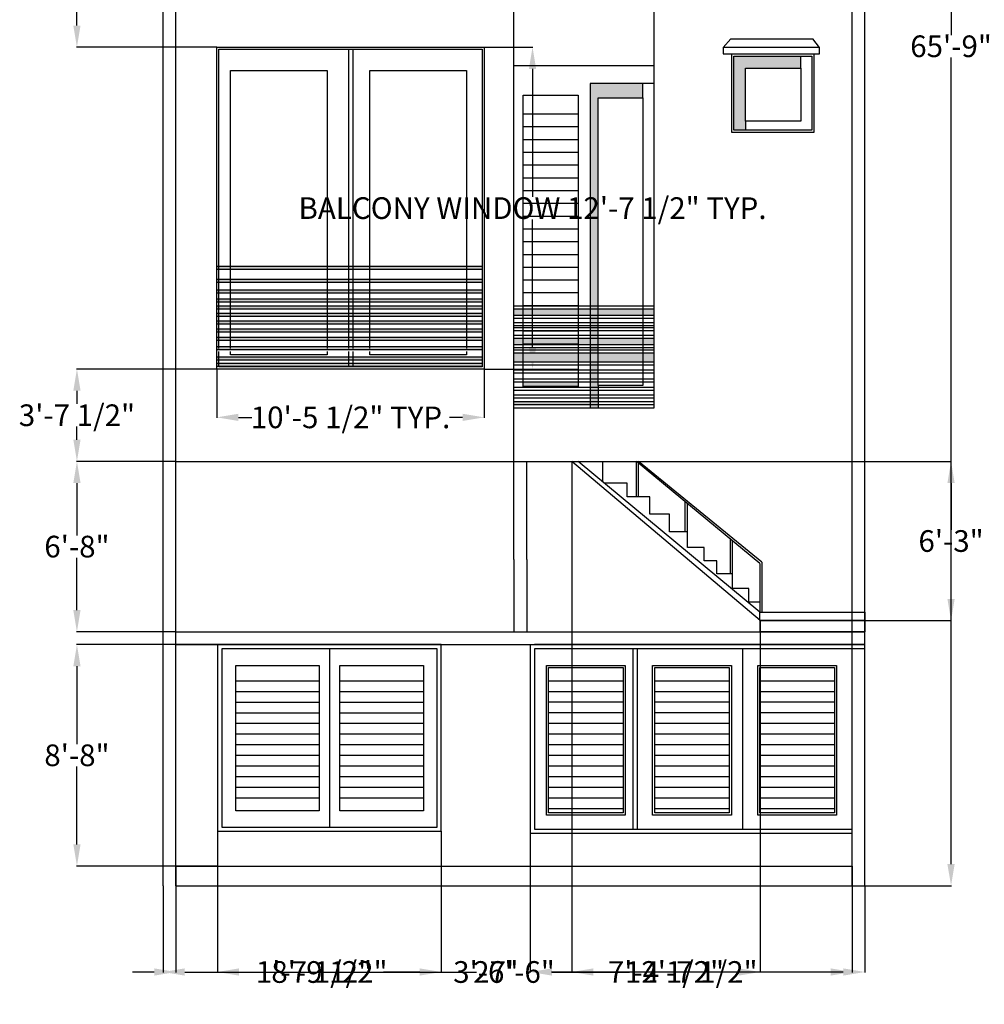
# Model space of a CAD drawing. Units: inches. Extents: x 41 to 5965, y 7 to 3328.
# Tile 4 of 6: x 4990 to 5444, y 2428 to 2890. Entities that reach past the tile are written whole.
import ezdxf

# ---------------------------------------------------------------- set-up
doc = ezdxf.new("R2010")
doc.units = ezdxf.units.IN
doc.header["$MEASUREMENT"] = 0
for name, color, linetype, lineweight in [('A-ANNO-DIMS', 2, 'Continuous', 18), ('A-ELEV', 7, 'Continuous', 25), ('A-ELEV-PATT', 8, 'Continuous', 13)]:
    doc.layers.add(name, color=color, linetype=linetype, lineweight=lineweight)
doc.styles.get("Standard").update_dxf_attribs({"font": 'arial.ttf'})
doc.dimstyles.get("Standard").update_dxf_attribs({"dimtxt": 10.18, "dimasz": 10.18, "dimexe": 0.18, "dimexo": 0.0625, "dimgap": 0.09, "dimtad": 0, "dimtih": 1, "dimtoh": 1, "dimdec": 0, "dimzin": 0, "dimdsep": 46, "dimlunit": 3, "dimtxsty": 'Standard', "dimcen": 0.09, "dimadec": 0, "dimazin": 0, "dimtfac": 1, "dimtdec": 0, "dimtofl": 0, "dimtmove": 0, "dimatfit": 3, "dimfxl": 1, "dimtolj": 1, "dimtzin": 0, "dimarcsym": 0})

# ---------------------------------------------------------------- blocks, each defined once
blk = doc.blocks.new('WIN-ELEV-1')
for p, q in [((0, 0), (0, 151.25)), ((0, 151.25), (125.74, 151.25)), ((1, 150.25), (124.74, 150.25)), ((1, 9.67), (1, 150.25)), ((124.74, 150.25), (124.74, 1)), ((125.74, 151.25), (125.74, 0)), ((1, 1), (1, 8.26)), ((125.74, 0), (0, 0)), ((124.74, 1), (1, 1))]:
    blk.add_line(p, q)
blk = doc.blocks.new('*D32')
at = {"layer": 'A-ANNO-DIMS', "color": 0, "lineweight": -2, "transparency": 16777216}
for p, q in [((5208.81, 2877.58), (5231.61, 2877.58)), ((5231.43, 2867.4), (5231.43, 2807.31)), ((5231.43, 2736.51), (5231.43, 2796.6)), ((5208.81, 2726.33), (5231.61, 2726.33))]:
    blk.add_line(p, q, dxfattribs=at)
at = {"layer": 'A-ANNO-DIMS', "color": 0, "transparency": 16777216}
for points in [[(5229.74, 2867.4), (5233.13, 2867.4), (5231.43, 2877.58)], [(5229.74, 2736.51), (5233.13, 2736.51), (5231.43, 2726.33)]]:
    blk.add_solid(points, dxfattribs=at)
at = {"layer": 'Defpoints', "color": 0, "transparency": 16777216}
for p in [(5208.74, 2877.58), (5231.43, 2877.58), (5208.74, 2726.33)]:
    blk.add_point(p, dxfattribs=at)
at = {"layer": 'A-ANNO-DIMS', "color": 0, "transparency": 16777216, "insert": (5231.43, 2801.96), "char_height": 10.18, "attachment_point": 5}
blk.add_mtext('\\A1;BALCONY WINDOW 12\'-7 1/2" TYP.', dxfattribs=at)
blk = doc.blocks.new('*D33')
at = {"layer": 'A-ANNO-DIMS', "color": 0, "lineweight": -2, "transparency": 16777216}
for p, q in [((5083, 2726.27), (5083, 2703.46)), ((5208.74, 2726.27), (5208.74, 2703.46)), ((5093.18, 2703.64), (5099.42, 2703.64)), ((5198.56, 2703.64), (5192.33, 2703.64))]:
    blk.add_line(p, q, dxfattribs=at)
at = {"layer": 'A-ANNO-DIMS', "color": 0, "transparency": 16777216}
for points in [[(5093.18, 2705.34), (5093.18, 2701.95), (5083, 2703.64)], [(5198.56, 2705.34), (5198.56, 2701.95), (5208.74, 2703.64)]]:
    blk.add_solid(points, dxfattribs=at)
at = {"layer": 'Defpoints', "color": 0, "transparency": 16777216}
for p in [(5083, 2726.33), (5208.74, 2726.33), (5208.74, 2703.64)]:
    blk.add_point(p, dxfattribs=at)
at = {"layer": 'A-ANNO-DIMS', "color": 0, "transparency": 16777216, "insert": (5145.87, 2703.64), "char_height": 10.18, "attachment_point": 5}
blk.add_mtext('\\A1;10\'-5 1/2" TYP.', dxfattribs=at)
blk = doc.blocks.new('*D63')
at = {"layer": 'A-ANNO-DIMS', "color": 0, "lineweight": -2, "transparency": 16777216}
for p, q in [((5057.72, 2483.48), (5057.72, 2442.86)), ((5387.72, 2483.48), (5387.72, 2442.86)), ((5067.9, 2443.04), (5205.06, 2443.04)), ((5377.54, 2443.04), (5240.38, 2443.04))]:
    blk.add_line(p, q, dxfattribs=at)
at = {"layer": 'A-ANNO-DIMS', "color": 0, "transparency": 16777216}
for points in [[(5067.9, 2444.74), (5067.9, 2441.34), (5057.72, 2443.04)], [(5377.54, 2444.74), (5377.54, 2441.34), (5387.72, 2443.04)]]:
    blk.add_solid(points, dxfattribs=at)
at = {"layer": 'Defpoints', "color": 0, "transparency": 16777216}
for p in [(5057.72, 2483.54), (5387.72, 2483.54), (5387.72, 2443.04)]:
    blk.add_point(p, dxfattribs=at)
at = {"layer": 'A-ANNO-DIMS', "color": 0, "transparency": 16777216, "insert": (5222.72, 2443.04), "char_height": 10.18, "attachment_point": 5}
blk.add_mtext('\\A1;27\'-6"', dxfattribs=at)
blk = doc.blocks.new('*D64')
at = {"layer": 'A-ANNO-DIMS', "color": 0, "lineweight": -2, "transparency": 16777216}
for p, q in [((5387.78, 3272.46), (5428.4, 3272.46)), ((5428.22, 3262.28), (5428.22, 2883.29)), ((5428.22, 2493.72), (5428.22, 2872.71)), ((5387.78, 2483.54), (5428.4, 2483.54))]:
    blk.add_line(p, q, dxfattribs=at)
at = {"layer": 'A-ANNO-DIMS', "color": 0, "transparency": 16777216}
for points in [[(5426.52, 3262.28), (5429.92, 3262.28), (5428.22, 3272.46)], [(5426.52, 2493.72), (5429.92, 2493.72), (5428.22, 2483.54)]]:
    blk.add_solid(points, dxfattribs=at)
at = {"layer": 'Defpoints', "color": 0, "transparency": 16777216}
for p in [(5387.72, 3272.46), (5428.22, 3272.46), (5387.72, 2483.54)]:
    blk.add_point(p, dxfattribs=at)
at = {"layer": 'A-ANNO-DIMS', "color": 0, "transparency": 16777216, "insert": (5428.22, 2878), "char_height": 10.18, "attachment_point": 5}
blk.add_mtext('\\A1;65\'-9"', dxfattribs=at)
blk = doc.blocks.new('*D65')
at = {"layer": 'A-ANNO-DIMS', "color": 0, "lineweight": -2, "transparency": 16777216}
for p, q in [((5063.72, 2492.78), (5063.72, 2442.86)), ((5083.3, 2492.78), (5083.3, 2442.86)), ((5053.54, 2443.04), (5043.36, 2443.04)), ((5093.48, 2443.04), (5103.66, 2443.04))]:
    blk.add_line(p, q, dxfattribs=at)
at = {"layer": 'A-ANNO-DIMS', "color": 0, "transparency": 16777216}
for points in [[(5053.54, 2444.74), (5053.54, 2441.34), (5063.72, 2443.04)], [(5093.48, 2444.74), (5093.48, 2441.34), (5083.3, 2443.04)]]:
    blk.add_solid(points, dxfattribs=at)
at = {"layer": 'Defpoints', "color": 0, "transparency": 16777216}
for p in [(5063.72, 2492.84), (5083.3, 2492.84), (5083.3, 2443.04)]:
    blk.add_point(p, dxfattribs=at)
at = {"layer": 'A-ANNO-DIMS', "color": 0, "transparency": 16777216, "insert": (5128.66, 2443.04), "char_height": 10.18, "attachment_point": 5}
blk.add_mtext('\\A1;1\'-7 1/2"', dxfattribs=at)
blk = doc.blocks.new('*D66')
at = {"layer": 'A-ANNO-DIMS', "color": 0, "lineweight": -2, "transparency": 16777216}
for p, q in [((5083.3, 2492.78), (5083.3, 2442.86)), ((5188.55, 2492.78), (5188.55, 2442.86)), ((5093.48, 2443.04), (5110.44, 2443.04)), ((5178.37, 2443.04), (5161.41, 2443.04))]:
    blk.add_line(p, q, dxfattribs=at)
at = {"layer": 'A-ANNO-DIMS', "color": 0, "transparency": 16777216}
for points in [[(5093.48, 2444.74), (5093.48, 2441.34), (5083.3, 2443.04)], [(5178.37, 2444.74), (5178.37, 2441.34), (5188.55, 2443.04)]]:
    blk.add_solid(points, dxfattribs=at)
at = {"layer": 'Defpoints', "color": 0, "transparency": 16777216}
for p in [(5083.3, 2492.84), (5188.55, 2492.84), (5188.55, 2443.04)]:
    blk.add_point(p, dxfattribs=at)
at = {"layer": 'A-ANNO-DIMS', "color": 0, "transparency": 16777216, "insert": (5135.93, 2443.04), "char_height": 10.18, "attachment_point": 5}
blk.add_mtext('\\A1;8\'-9 1/2"', dxfattribs=at)
blk = doc.blocks.new('*D67')
at = {"layer": 'A-ANNO-DIMS', "color": 0, "lineweight": -2, "transparency": 16777216}
for p, q in [((5188.55, 2492.78), (5188.55, 2442.86)), ((5230.39, 2492.78), (5230.39, 2442.86)), ((5178.37, 2443.04), (5168.19, 2443.04)), ((5240.57, 2443.04), (5250.75, 2443.04))]:
    blk.add_line(p, q, dxfattribs=at)
at = {"layer": 'A-ANNO-DIMS', "color": 0, "transparency": 16777216}
for points in [[(5178.37, 2444.74), (5178.37, 2441.34), (5188.55, 2443.04)], [(5240.57, 2444.74), (5240.57, 2441.34), (5230.39, 2443.04)]]:
    blk.add_solid(points, dxfattribs=at)
at = {"layer": 'Defpoints', "color": 0, "transparency": 16777216}
for p in [(5188.55, 2492.84), (5230.39, 2492.84), (5230.39, 2443.04)]:
    blk.add_point(p, dxfattribs=at)
at = {"layer": 'A-ANNO-DIMS', "color": 0, "transparency": 16777216, "insert": (5209.47, 2443.04), "char_height": 10.18, "attachment_point": 5}
blk.add_mtext('\\A1;3\'-6"', dxfattribs=at)
blk = doc.blocks.new('*D68')
at = {"layer": 'A-ANNO-DIMS', "color": 0, "lineweight": -2, "transparency": 16777216}
for p, q in [((5230.39, 2492.78), (5230.39, 2442.86)), ((5381.72, 2492.78), (5381.72, 2442.86)), ((5240.57, 2443.04), (5277.1, 2443.04)), ((5371.54, 2443.04), (5335.01, 2443.04))]:
    blk.add_line(p, q, dxfattribs=at)
at = {"layer": 'A-ANNO-DIMS', "color": 0, "transparency": 16777216}
for points in [[(5240.57, 2444.74), (5240.57, 2441.34), (5230.39, 2443.04)], [(5371.54, 2444.74), (5371.54, 2441.34), (5381.72, 2443.04)]]:
    blk.add_solid(points, dxfattribs=at)
at = {"layer": 'Defpoints', "color": 0, "transparency": 16777216}
for p in [(5230.39, 2492.84), (5381.72, 2492.84), (5381.72, 2443.04)]:
    blk.add_point(p, dxfattribs=at)
at = {"layer": 'A-ANNO-DIMS', "color": 0, "transparency": 16777216, "insert": (5306.06, 2443.04), "char_height": 10.18, "attachment_point": 5}
blk.add_mtext('\\A1;12\'-7 1/2"', dxfattribs=at)
blk = doc.blocks.new('*D69')
at = {"layer": 'A-ANNO-DIMS', "color": 0, "lineweight": -2, "transparency": 16777216}
for p, q in [((5083.23, 2596.88), (5017.04, 2596.88)), ((5017.22, 2586.7), (5017.22, 2550.15)), ((5017.22, 2503.02), (5017.22, 2539.57)), ((5083.23, 2492.84), (5017.04, 2492.84))]:
    blk.add_line(p, q, dxfattribs=at)
at = {"layer": 'A-ANNO-DIMS', "color": 0, "transparency": 16777216}
for points in [[(5015.52, 2586.7), (5018.92, 2586.7), (5017.22, 2596.88)], [(5015.52, 2503.02), (5018.92, 2503.02), (5017.22, 2492.84)]]:
    blk.add_solid(points, dxfattribs=at)
at = {"layer": 'Defpoints', "color": 0, "transparency": 16777216}
for p in [(5017.22, 2596.88), (5083.3, 2596.88), (5083.3, 2492.84)]:
    blk.add_point(p, dxfattribs=at)
at = {"layer": 'A-ANNO-DIMS', "color": 0, "transparency": 16777216, "insert": (5017.22, 2544.86), "char_height": 10.18, "attachment_point": 5}
blk.add_mtext('\\A1;8\'-8"', dxfattribs=at)
blk = doc.blocks.new('*D70')
at = {"layer": 'A-ANNO-DIMS', "color": 0, "lineweight": -2, "transparency": 16777216}
for p, q in [((5063.66, 2682.95), (5017.04, 2682.95)), ((5017.22, 2672.77), (5017.22, 2648.2)), ((5017.22, 2613.06), (5017.22, 2637.63)), ((5063.66, 2602.88), (5017.04, 2602.88))]:
    blk.add_line(p, q, dxfattribs=at)
at = {"layer": 'A-ANNO-DIMS', "color": 0, "transparency": 16777216}
for points in [[(5015.52, 2672.77), (5018.92, 2672.77), (5017.22, 2682.95)], [(5015.52, 2613.06), (5018.92, 2613.06), (5017.22, 2602.88)]]:
    blk.add_solid(points, dxfattribs=at)
at = {"layer": 'Defpoints', "color": 0, "transparency": 16777216}
for p in [(5017.22, 2682.95), (5063.72, 2682.95), (5063.72, 2602.88)]:
    blk.add_point(p, dxfattribs=at)
at = {"layer": 'A-ANNO-DIMS', "color": 0, "transparency": 16777216, "insert": (5017.22, 2642.92), "char_height": 10.18, "attachment_point": 5}
blk.add_mtext('\\A1;6\'-8"', dxfattribs=at)
blk = doc.blocks.new('*D71')
at = {"layer": 'A-ANNO-DIMS', "color": 0, "lineweight": -2, "transparency": 16777216}
for p, q in [((5082.94, 2726.33), (5017.04, 2726.33)), ((5017.22, 2716.15), (5017.22, 2710)), ((5017.22, 2693.13), (5017.22, 2699.28)), ((5063.66, 2682.95), (5017.04, 2682.95))]:
    blk.add_line(p, q, dxfattribs=at)
at = {"layer": 'A-ANNO-DIMS', "color": 0, "transparency": 16777216}
for points in [[(5015.52, 2716.15), (5018.92, 2716.15), (5017.22, 2726.33)], [(5015.52, 2693.13), (5018.92, 2693.13), (5017.22, 2682.95)]]:
    blk.add_solid(points, dxfattribs=at)
at = {"layer": 'Defpoints', "color": 0, "transparency": 16777216}
for p in [(5017.22, 2726.33), (5083, 2726.33), (5063.72, 2682.95)]:
    blk.add_point(p, dxfattribs=at)
at = {"layer": 'A-ANNO-DIMS', "color": 0, "transparency": 16777216, "insert": (5017.22, 2704.64), "char_height": 10.18, "attachment_point": 5}
blk.add_mtext('\\A1;3\'-7 1/2"', dxfattribs=at)
blk = doc.blocks.new('*D72')
at = {"layer": 'A-ANNO-DIMS', "color": 0, "lineweight": -2, "transparency": 16777216}
for p, q in [((5079.42, 2985.67), (5017.04, 2985.67)), ((5017.22, 2975.49), (5017.22, 2936.92)), ((5017.22, 2887.76), (5017.22, 2926.34)), ((5082.94, 2877.58), (5017.04, 2877.58))]:
    blk.add_line(p, q, dxfattribs=at)
at = {"layer": 'A-ANNO-DIMS', "color": 0, "transparency": 16777216}
for points in [[(5015.52, 2975.49), (5018.92, 2975.49), (5017.22, 2985.67)], [(5015.52, 2887.76), (5018.92, 2887.76), (5017.22, 2877.58)]]:
    blk.add_solid(points, dxfattribs=at)
at = {"layer": 'Defpoints', "color": 0, "transparency": 16777216}
for p in [(5017.22, 2985.67), (5079.49, 2985.67), (5083, 2877.58)]:
    blk.add_point(p, dxfattribs=at)
at = {"layer": 'A-ANNO-DIMS', "color": 0, "transparency": 16777216, "insert": (5017.22, 2931.63), "char_height": 10.18, "attachment_point": 5}
blk.add_mtext('\\A1;9\'-0"', dxfattribs=at)
blk = doc.blocks.new('*D77')
at = {"layer": 'A-ANNO-DIMS', "color": 0, "lineweight": -2, "transparency": 16777216}
for p, q in [((5249.9, 2682.89), (5249.9, 2442.86)), ((5338.47, 2608.06), (5338.47, 2442.86)), ((5260.08, 2443.04), (5268.75, 2443.04)), ((5328.29, 2443.04), (5319.63, 2443.04))]:
    blk.add_line(p, q, dxfattribs=at)
at = {"layer": 'A-ANNO-DIMS', "color": 0, "transparency": 16777216}
for points in [[(5260.08, 2444.74), (5260.08, 2441.34), (5249.9, 2443.04)], [(5328.29, 2444.74), (5328.29, 2441.34), (5338.47, 2443.04)]]:
    blk.add_solid(points, dxfattribs=at)
at = {"layer": 'Defpoints', "color": 0, "transparency": 16777216}
for p in [(5249.9, 2682.95), (5338.47, 2608.13), (5338.47, 2443.04)]:
    blk.add_point(p, dxfattribs=at)
at = {"layer": 'A-ANNO-DIMS', "color": 0, "transparency": 16777216, "insert": (5294.19, 2443.04), "char_height": 10.18, "attachment_point": 5}
blk.add_mtext('\\A1;7\'-4 1/2"', dxfattribs=at)
blk = doc.blocks.new('*D78')
at = {"layer": 'A-ANNO-DIMS', "color": 0, "lineweight": -2, "transparency": 16777216}
for p, q in [((5249.96, 2682.95), (5428.4, 2682.95)), ((5428.22, 2672.77), (5428.22, 2650.83)), ((5428.22, 2618.31), (5428.22, 2640.25)), ((5338.54, 2608.13), (5428.4, 2608.13))]:
    blk.add_line(p, q, dxfattribs=at)
at = {"layer": 'A-ANNO-DIMS', "color": 0, "transparency": 16777216}
for points in [[(5426.52, 2672.77), (5429.92, 2672.77), (5428.22, 2682.95)], [(5426.52, 2618.31), (5429.92, 2618.31), (5428.22, 2608.13)]]:
    blk.add_solid(points, dxfattribs=at)
at = {"layer": 'Defpoints', "color": 0, "transparency": 16777216}
for p in [(5249.9, 2682.95), (5338.47, 2608.13), (5428.22, 2608.13)]:
    blk.add_point(p, dxfattribs=at)
at = {"layer": 'A-ANNO-DIMS', "color": 0, "transparency": 16777216, "insert": (5428.22, 2645.54), "char_height": 10.18, "attachment_point": 5}
blk.add_mtext('\\A1;6\'-3"', dxfattribs=at)

msp = doc.modelspace()

# ---------------------------------------------------------------- hatches: boundary and pattern name
at = {"layer": 'A-ELEV-PATT'}
h = msp.add_hatch(color=256, dxfattribs=at)
h.dxf.hatch_style = 1
h.paths.add_polyline_path([(5326.1, 2838.56), (5331.59, 2838.56), (5331.59, 2842.77), (5331.59, 2867.75), (5357.62, 2867.75), (5357.62, 2873.38), (5326.1, 2873.38)])
h = msp.add_hatch(color=256, dxfattribs=at)
h.dxf.hatch_style = 1
h.paths.add_polyline_path([(5283.31, 2860.46), (5258.54, 2860.46), (5258.54, 2708.16), (5262.29, 2708.16), (5262.29, 2718.67), (5262.29, 2853.73), (5283.31, 2853.73)])
h = msp.add_hatch(color=256, dxfattribs=at)
h.dxf.hatch_style = 1
h.paths.add_polyline_path([(5207.74, 2774.65), (5083, 2774.65), (5083, 2773.25), (5207.74, 2773.25)])
h = msp.add_hatch(color=256, dxfattribs=at)
h.dxf.hatch_style = 1
h.paths.add_polyline_path([(5207.74, 2768.59), (5083, 2768.59), (5083, 2767.18), (5207.74, 2767.18)])
h = msp.add_hatch(color=256, dxfattribs=at)
h.dxf.hatch_style = 1
h.paths.add_polyline_path([(5207.74, 2763.59), (5083, 2763.59), (5083, 2762.18), (5207.74, 2762.18)])
h = msp.add_hatch(color=256, dxfattribs=at)
h.dxf.hatch_style = 1
h.paths.add_polyline_path([(5207.74, 2759.3), (5083, 2759.3), (5083, 2757.89), (5207.74, 2757.89)])
h = msp.add_hatch(color=256, dxfattribs=at)
h.dxf.hatch_style = 1
h.paths.add_polyline_path([(5207.74, 2756.07), (5083, 2756.07), (5083, 2754.67), (5207.74, 2754.67)])
h = msp.add_hatch(color=256, dxfattribs=at)
h.dxf.hatch_style = 1
h.paths.add_polyline_path([(5252.94, 2740.84), (5227.05, 2740.84), (5227.05, 2738.24), (5252.94, 2738.24)])
h.paths.add_polyline_path([(5227.05, 2740.84), (5222.72, 2740.84), (5222.72, 2737.95), (5227.05, 2737.95)])
h.paths.add_polyline_path([(5283.31, 2740.84), (5262.29, 2740.84), (5262.29, 2737.95), (5283.31, 2737.95)])
h.paths.add_polyline_path([(5258.54, 2740.84), (5252.94, 2740.84), (5252.94, 2737.95), (5258.54, 2737.95)])
h.paths.add_polyline_path([(5288.65, 2740.84), (5283.31, 2740.84), (5283.31, 2737.95), (5288.65, 2737.95)])
h.paths.add_polyline_path([(5283.31, 2754.66), (5262.29, 2754.66), (5262.29, 2751.62), (5283.31, 2751.62)])
h.paths.add_polyline_path([(5252.94, 2754.66), (5227.05, 2754.66), (5227.05, 2751.62), (5252.94, 2751.62)])
h.paths.add_polyline_path([(5258.54, 2754.66), (5252.94, 2754.66), (5252.94, 2751.62), (5258.54, 2751.62)])
h.paths.add_polyline_path([(5288.65, 2754.66), (5283.31, 2754.66), (5283.31, 2751.62), (5288.65, 2751.62)])
h.paths.add_polyline_path([(5227.05, 2754.66), (5222.72, 2754.66), (5222.72, 2751.62), (5227.05, 2751.62)])
h.paths.add_polyline_path([(5283.31, 2733.93), (5262.29, 2733.93), (5262.29, 2729.81), (5283.31, 2729.81)])
h = msp.add_hatch(color=256, dxfattribs=at)
h.dxf.hatch_style = 1
h.paths.add_polyline_path([(5207.74, 2752.65), (5083, 2752.65), (5083, 2751.24), (5207.74, 2751.24)])
h = msp.add_hatch(color=256, dxfattribs=at)
h.dxf.hatch_style = 1
h.paths.add_polyline_path([(5207.74, 2748.99), (5083, 2748.99), (5083, 2747.59), (5207.74, 2747.59)])
h = msp.add_hatch(color=256, dxfattribs=at)
h.dxf.hatch_style = 1
h.paths.add_polyline_path([(5207.74, 2745.19), (5083, 2745.19), (5083, 2743.79), (5207.74, 2743.79)])
h = msp.add_hatch(color=256, dxfattribs=at)
h.dxf.hatch_style = 1
h.paths.add_polyline_path([(5207.74, 2741.28), (5083, 2741.28), (5083, 2739.87), (5207.74, 2739.87)])
h = msp.add_hatch(color=256, dxfattribs=at)
h.dxf.hatch_style = 1
h.paths.add_polyline_path([(5207.74, 2737), (5083, 2737), (5083, 2735.59), (5207.74, 2735.59)])
h = msp.add_hatch(color=256, dxfattribs=at)
h.dxf.hatch_style = 1
h.paths.add_polyline_path([(5207.74, 2732.1), (5083, 2732.1), (5083, 2730.69), (5207.74, 2730.69)])
h = msp.add_hatch(color=256, dxfattribs=at)
h.dxf.hatch_style = 1
h.paths.add_polyline_path([(5252.94, 2733.93), (5227.05, 2733.93), (5227.05, 2729.81), (5252.94, 2729.81)])
h.paths.add_polyline_path([(5227.05, 2733.93), (5222.72, 2733.93), (5222.72, 2729.81), (5227.05, 2729.81)])
h.paths.add_polyline_path([(5258.54, 2733.93), (5252.94, 2733.93), (5252.94, 2729.81), (5258.54, 2729.81)])
h.paths.add_polyline_path([(5288.65, 2733.93), (5283.31, 2733.93), (5283.31, 2729.81), (5288.65, 2729.81)])
h.paths.add_polyline_path([(5252.94, 2720.41), (5227.05, 2720.41), (5227.05, 2718.13), (5252.94, 2718.13)])
h.paths.add_polyline_path([(5258.54, 2711.07), (5222.72, 2711.07), (5222.72, 2709.66), (5258.54, 2709.66)])
h = msp.add_hatch(color=256, dxfattribs=at)
h.dxf.hatch_style = 1
h.paths.add_polyline_path([(5207.74, 2729.18), (5083, 2729.18), (5083, 2727.77), (5207.74, 2727.77)])

# ---------------------------------------------------------------- linework, layer by layer
at = {"layer": 'A-ELEV'}
for p, q in [((5057.72, 2483.54), (5057.72, 3272.46)), ((5222.72, 2682.95), (5222.72, 3272.46)), ((5288.65, 2708.16), (5288.65, 3272.46)), ((5381.72, 2483.54), (5381.72, 3272.46)), ((5387.72, 2483.54), (5387.72, 3272.46)), ((5063.72, 2483.54), (5063.72, 3263.67)), ((5321.09, 2877.43), (5324.61, 2881.49)), ((5324.61, 2881.49), (5363.21, 2881.49)), ((5366.37, 2877.43), (5363.21, 2881.49)), ((5144.87, 2876.58), (5144.87, 2736)), ((5146.87, 2876.58), (5146.87, 2736)), ((5357.62, 2867.75), (5357.62, 2873.38)), ((5222.72, 2868.96), (5288.65, 2868.96)), ((5288.65, 2860.46), (5258.54, 2860.46)), ((5258.54, 2860.46), (5258.54, 2708.16)), ((5283.31, 2853.73), (5283.31, 2860.46)), ((5227.05, 2846.24), (5252.94, 2846.24)), ((5331.59, 2842.77), (5331.59, 2838.56)), ((5227.05, 2840.24), (5252.94, 2840.24)), ((5227.05, 2834.24), (5252.94, 2834.24)), ((5227.05, 2828.24), (5252.94, 2828.24)), ((5227.05, 2822.24), (5252.94, 2822.24)), ((5227.05, 2816.24), (5252.94, 2816.24)), ((5227.05, 2810.24), (5252.94, 2810.24)), ((5227.05, 2804.24), (5252.94, 2804.24)), ((5227.05, 2798.24), (5252.94, 2798.24)), ((5227.05, 2792.24), (5252.94, 2792.24)), ((5227.05, 2786.24), (5252.94, 2786.24)), ((5227.05, 2780.24), (5252.94, 2780.24)), ((5083, 2774.65), (5207.74, 2774.65)), ((5083, 2773.25), (5207.74, 2773.25)), ((5227.05, 2774.24), (5252.94, 2774.24)), ((5083, 2768.59), (5207.74, 2768.59)), ((5083, 2767.18), (5207.74, 2767.18)), ((5227.05, 2768.24), (5252.94, 2768.24)), ((5083, 2763.59), (5207.74, 2763.59)), ((5083, 2762.18), (5207.74, 2762.18)), ((5227.05, 2762.24), (5252.94, 2762.24)), ((5083, 2759.3), (5207.74, 2759.3)), ((5083, 2757.89), (5207.74, 2757.89)), ((5083, 2756.07), (5207.74, 2756.07)), ((5083, 2754.67), (5207.74, 2754.67)), ((5222.72, 2756.07), (5288.65, 2756.07)), ((5222.72, 2754.66), (5288.65, 2754.66)), ((5227.05, 2756.24), (5252.94, 2756.24)), ((5083, 2752.65), (5207.74, 2752.65)), ((5083, 2751.24), (5207.74, 2751.24)), ((5083, 2748.99), (5207.74, 2748.99)), ((5222.72, 2751.62), (5288.65, 2751.62)), ((5222.72, 2750.21), (5288.65, 2750.21)), ((5222.72, 2748.24), (5288.65, 2748.24)), ((5227.05, 2750.24), (5252.94, 2750.24)), ((5083, 2747.59), (5207.74, 2747.59)), ((5083, 2745.19), (5207.74, 2745.19)), ((5083, 2743.79), (5207.74, 2743.79)), ((5222.72, 2746.83), (5288.65, 2746.83)), ((5222.72, 2745.94), (5288.65, 2745.94)), ((5222.72, 2744.53), (5288.65, 2744.53)), ((5227.05, 2744.24), (5252.94, 2744.24)), ((5083, 2741.28), (5207.74, 2741.28)), ((5083, 2739.87), (5207.74, 2739.87)), ((5222.72, 2742.25), (5288.65, 2742.25)), ((5222.72, 2740.84), (5288.65, 2740.84)), ((5083, 2737), (5207.74, 2737)), ((5083, 2735.59), (5207.74, 2735.59)), ((5144.87, 2734.59), (5144.87, 2727.33)), ((5146.87, 2734.59), (5146.87, 2727.33)), ((5222.72, 2737.95), (5288.65, 2737.95)), ((5222.72, 2736.54), (5288.65, 2736.54)), ((5222.72, 2735.34), (5288.65, 2735.34)), ((5227.05, 2738.24), (5252.94, 2738.24)), ((5083, 2732.1), (5207.74, 2732.1)), ((5083, 2730.69), (5207.74, 2730.69)), ((5222.72, 2733.93), (5288.65, 2733.93)), ((5222.72, 2729.81), (5288.65, 2729.81)), ((5083, 2729.18), (5207.74, 2729.18)), ((5083, 2727.77), (5207.74, 2727.77)), ((5222.72, 2728.4), (5288.65, 2728.4)), ((5222.72, 2725.97), (5288.65, 2725.97)), ((5227.05, 2726.24), (5252.94, 2726.24)), ((5222.72, 2724.56), (5288.65, 2724.56)), ((5222.72, 2721.82), (5288.65, 2721.82)), ((5222.72, 2720.41), (5288.65, 2720.41)), ((5222.72, 2717.83), (5288.65, 2717.83)), ((5222.72, 2716.42), (5288.65, 2716.42)), ((5262.29, 2718.67), (5262.29, 2708.16)), ((5222.72, 2714.3), (5288.65, 2714.3)), ((5222.72, 2712.89), (5288.65, 2712.89)), ((5222.72, 2711.07), (5288.65, 2711.07)), ((5222.72, 2709.66), (5288.65, 2709.66)), ((5222.72, 2708.16), (5288.65, 2708.16)), ((5063.72, 2682.95), (5387.72, 2682.95)), ((5222.72, 2636.84), (5222.72, 2682.95)), ((5228.72, 2636.84), (5228.72, 2682.95)), ((5338.47, 2608.13), (5249.9, 2682.95)), ((5338.25, 2612.15), (5252.82, 2682.95)), ((5264.53, 2673.25), (5264.53, 2682.95)), ((5280.26, 2666.28), (5280.26, 2682.95)), ((5338.25, 2635.02), (5280.26, 2682.95)), ((5281.26, 2666.28), (5281.26, 2682.95)), ((5339.32, 2635.64), (5281.26, 2682.95)), ((5303.25, 2682.95), (5303.25, 2683.13)), ((5304.25, 2682.95), (5304.25, 2683.13)), ((5275.92, 2672.69), (5265.2, 2672.69)), ((5275.92, 2666.28), (5275.92, 2672.69)), ((5286.61, 2666.28), (5275.92, 2666.28)), ((5286.61, 2658.22), (5286.61, 2666.28)), ((5303.25, 2649.82), (5303.25, 2663.95)), ((5304.25, 2649.82), (5304.25, 2663.13)), ((5295.88, 2658.22), (5286.61, 2658.22)), ((5295.88, 2649.82), (5295.88, 2658.22)), ((5304.25, 2649.82), (5295.88, 2649.82)), ((5304.25, 2642.56), (5304.25, 2649.82)), ((5324.51, 2630.09), (5324.51, 2646.38)), ((5312.16, 2642.56), (5304.25, 2642.56)), ((5312.16, 2636.25), (5312.16, 2642.56)), ((5325.51, 2630.09), (5325.51, 2645.55)), ((5222.72, 2636.84), (5222.72, 2602.88)), ((5228.72, 2636.84), (5228.72, 2602.88)), ((5318.05, 2636.25), (5312.16, 2636.25)), ((5318.05, 2630.09), (5318.05, 2636.25)), ((5338.25, 2635.02), (5338.25, 2612.15)), ((5339.32, 2635.64), (5339.32, 2612.15)), ((5325.51, 2630.09), (5318.05, 2630.09)), ((5325.51, 2623.21), (5325.51, 2630.09)), ((5333.11, 2623.21), (5325.51, 2623.21)), ((5333.11, 2616.77), (5333.11, 2623.21)), ((5338.25, 2616.77), (5333.11, 2616.77)), ((5063.72, 2602.88), (5387.72, 2602.88)), ((5063.72, 2596.88), (5387.72, 2596.88)), ((5083.3, 2596.88), (5083.3, 2509.14)), ((5188.55, 2596.88), (5083.3, 2596.88)), ((5188.55, 2509.14), (5188.55, 2596.88)), ((5230.39, 2596.88), (5230.39, 2492.84)), ((5387.72, 2596.88), (5232.39, 2596.88)), ((5085.3, 2594.88), (5085.3, 2511.14)), ((5186.55, 2594.88), (5085.3, 2594.88)), ((5135.93, 2594.88), (5135.93, 2511.14)), ((5186.55, 2511.14), (5186.55, 2594.88)), ((5232.39, 2594.88), (5232.39, 2510.22)), ((5387.72, 2594.88), (5232.39, 2594.88)), ((5278.76, 2510.22), (5278.76, 2594.88)), ((5280.76, 2510.22), (5280.76, 2594.88)), ((5330.17, 2594.88), (5330.17, 2510.22)), ((5381.72, 2483.54), (5381.72, 2594.88)), ((5381.72, 2508.22), (5381.72, 2594.88)), ((5381.72, 2492.84), (5381.72, 2594.88)), ((5091.87, 2579.88), (5131.15, 2579.88)), ((5140.86, 2579.88), (5180.14, 2579.88)), ((5238.99, 2579.91), (5274.06, 2579.91)), ((5288.88, 2579.91), (5323.94, 2579.91)), ((5338.3, 2579.91), (5373.36, 2579.91)), ((5091.87, 2574.88), (5131.15, 2574.88)), ((5140.86, 2574.88), (5180.14, 2574.88)), ((5238.99, 2574.91), (5274.06, 2574.91)), ((5288.88, 2574.91), (5323.94, 2574.91)), ((5338.3, 2574.91), (5373.36, 2574.91)), ((5091.87, 2569.88), (5131.15, 2569.88)), ((5140.86, 2569.88), (5180.14, 2569.88)), ((5238.99, 2569.91), (5274.06, 2569.91)), ((5288.88, 2569.91), (5323.94, 2569.91)), ((5338.3, 2569.91), (5373.36, 2569.91)), ((5091.87, 2564.88), (5131.15, 2564.88)), ((5140.86, 2564.88), (5180.14, 2564.88)), ((5238.99, 2564.91), (5274.06, 2564.91)), ((5288.88, 2564.91), (5323.94, 2564.91)), ((5338.3, 2564.91), (5373.36, 2564.91)), ((5091.87, 2559.88), (5131.15, 2559.88)), ((5140.86, 2559.88), (5180.14, 2559.88)), ((5238.99, 2559.91), (5274.06, 2559.91)), ((5288.88, 2559.91), (5323.94, 2559.91)), ((5338.3, 2559.91), (5373.36, 2559.91)), ((5091.87, 2554.88), (5131.15, 2554.88)), ((5140.86, 2554.88), (5180.14, 2554.88)), ((5238.99, 2554.91), (5274.06, 2554.91)), ((5288.88, 2554.91), (5323.94, 2554.91)), ((5338.3, 2554.91), (5373.36, 2554.91)), ((5091.87, 2549.88), (5131.15, 2549.88)), ((5140.86, 2549.88), (5180.14, 2549.88)), ((5238.99, 2549.91), (5274.06, 2549.91)), ((5288.88, 2549.91), (5323.94, 2549.91)), ((5338.3, 2549.91), (5373.36, 2549.91)), ((5091.87, 2544.88), (5131.15, 2544.88)), ((5140.86, 2544.88), (5180.14, 2544.88)), ((5238.99, 2544.91), (5274.06, 2544.91)), ((5288.88, 2544.91), (5323.94, 2544.91)), ((5338.3, 2544.91), (5373.36, 2544.91)), ((5091.87, 2539.88), (5131.15, 2539.88)), ((5140.86, 2539.88), (5180.14, 2539.88)), ((5238.99, 2539.91), (5274.06, 2539.91)), ((5288.88, 2539.91), (5323.94, 2539.91)), ((5338.3, 2539.91), (5373.36, 2539.91)), ((5091.87, 2534.88), (5131.15, 2534.88)), ((5140.86, 2534.88), (5180.14, 2534.88)), ((5238.99, 2534.91), (5274.06, 2534.91)), ((5288.88, 2534.91), (5323.94, 2534.91)), ((5338.3, 2534.91), (5373.36, 2534.91)), ((5091.87, 2529.88), (5131.15, 2529.88)), ((5140.86, 2529.88), (5180.14, 2529.88)), ((5238.99, 2529.91), (5274.06, 2529.91)), ((5288.88, 2529.91), (5323.94, 2529.91)), ((5338.3, 2529.91), (5373.36, 2529.91)), ((5091.87, 2524.88), (5131.15, 2524.88)), ((5140.86, 2524.88), (5180.14, 2524.88)), ((5238.99, 2524.91), (5274.06, 2524.91)), ((5288.88, 2524.91), (5323.94, 2524.91)), ((5338.3, 2524.91), (5373.36, 2524.91)), ((5063.72, 2483.54), (5063.72, 2519.54)), ((5238.99, 2519.91), (5274.06, 2519.91)), ((5288.88, 2519.91), (5323.94, 2519.91)), ((5338.3, 2519.91), (5373.36, 2519.91)), ((5083.3, 2509.14), (5188.55, 2509.14)), ((5083.3, 2509.14), (5083.3, 2492.84)), ((5085.3, 2511.14), (5186.55, 2511.14)), ((5188.55, 2509.14), (5188.55, 2492.84)), ((5230.39, 2508.22), (5381.72, 2508.22)), ((5232.39, 2510.22), (5381.72, 2510.22)), ((5063.72, 2492.84), (5381.72, 2492.84)), ((5063.72, 2483.54), (5387.72, 2483.54))]:
    msp.add_line(p, q, dxfattribs=at)
for points in [[(5321.09, 2874.38), (5321.09, 2874.38), (5366.37, 2874.38), (5366.37, 2874.38), (5366.37, 2877.43), (5366.37, 2877.43), (5321.09, 2877.43), (5321.09, 2877.43)], [(5325.1, 2874.38), (5325.1, 2874.38), (5363.69, 2874.38), (5363.69, 2874.38), (5363.69, 2837.56), (5363.69, 2837.56), (5325.1, 2837.56), (5325.1, 2837.56)], [(5326.1, 2873.38), (5362.69, 2873.38), (5362.69, 2838.56), (5326.1, 2838.56)], [(5331.59, 2867.75), (5331.59, 2867.75), (5357.62, 2867.75), (5357.62, 2867.75), (5357.62, 2842.77), (5357.62, 2842.77), (5331.59, 2842.77), (5331.59, 2842.77)], [(5227.05, 2855), (5227.05, 2855), (5252.94, 2855), (5252.94, 2855), (5252.94, 2718.13), (5252.94, 2718.13), (5227.05, 2718.13), (5227.05, 2718.13)], [(5262.29, 2853.73), (5262.29, 2853.73), (5283.31, 2853.73), (5283.31, 2853.73), (5283.31, 2718.67), (5283.31, 2718.67), (5262.29, 2718.67), (5262.29, 2718.67)], [(5387.72, 2608.13), (5387.72, 2608.13), (5338.25, 2608.13), (5338.25, 2608.13), (5338.25, 2612.15), (5338.25, 2612.15), (5387.72, 2612.15), (5387.72, 2612.15)], [(5387.72, 2602.88), (5387.72, 2602.88), (5338.47, 2602.88), (5338.47, 2602.88), (5338.47, 2608.13), (5338.47, 2608.13), (5387.72, 2608.13), (5387.72, 2608.13)], [(5091.87, 2587.07), (5091.87, 2587.07), (5131.15, 2587.07), (5131.15, 2587.07), (5131.15, 2518.75), (5131.15, 2518.75), (5091.87, 2518.75), (5091.87, 2518.75)], [(5140.86, 2587.07), (5140.86, 2587.07), (5180.14, 2587.07), (5180.14, 2587.07), (5180.14, 2518.75), (5180.14, 2518.75), (5140.86, 2518.75), (5140.86, 2518.75)], [(5237.99, 2587.07), (5237.99, 2587.07), (5275.06, 2587.07), (5275.06, 2587.07), (5275.06, 2516.76), (5275.06, 2516.76), (5237.99, 2516.76), (5237.99, 2516.76)], [(5287.88, 2587.07), (5287.88, 2587.07), (5324.94, 2587.07), (5324.94, 2587.07), (5324.94, 2516.76), (5324.94, 2516.76), (5287.88, 2516.76), (5287.88, 2516.76)], [(5337.3, 2587.07), (5337.3, 2587.07), (5374.36, 2587.07), (5374.36, 2587.07), (5374.36, 2516.76), (5374.36, 2516.76), (5337.3, 2516.76), (5337.3, 2516.76)], [(5238.99, 2586.07), (5274.06, 2586.07), (5274.06, 2517.76), (5238.99, 2517.76)], [(5288.88, 2586.07), (5323.94, 2586.07), (5323.94, 2517.76), (5288.88, 2517.76)], [(5338.3, 2586.07), (5373.36, 2586.07), (5373.36, 2517.76), (5338.3, 2517.76)]]:
    msp.add_lwpolyline(points, close=True, dxfattribs=at)
for points in [[(5089.46, 2736), (5089.46, 2866.57), (5089.46, 2866.57), (5134.87, 2866.57), (5134.87, 2866.57), (5134.87, 2736)], [(5154.97, 2736), (5154.97, 2866.57), (5154.97, 2866.57), (5200.38, 2866.57), (5200.38, 2866.57), (5200.38, 2736)], [(5134.87, 2734.59), (5134.87, 2733.1), (5134.87, 2733.1), (5089.46, 2733.1), (5089.46, 2733.1), (5089.46, 2734.59)], [(5200.38, 2734.59), (5200.38, 2733.1), (5200.38, 2733.1), (5154.97, 2733.1), (5154.97, 2733.1), (5154.97, 2734.59)]]:
    msp.add_lwpolyline(points, dxfattribs=at)

# ---------------------------------------------------------------- block references
msp.add_blockref('WIN-ELEV-1', (5083, 2726.33), dxfattribs=at)

# ---------------------------------------------------------------- dimensions: what is measured, and where the dimension line sits
at = {"layer": 'A-ANNO-DIMS'}
for base, p1, p2, picture, middle in [((5428.22, 3272.46), (5387.72, 2483.54), (5387.72, 3272.46), '*D64', (5428.22, 2878)), ((5017.22, 2985.67), (5083, 2877.58), (5079.49, 2985.67), '*D72', (5017.22, 2931.63)), ((5017.22, 2726.33), (5063.72, 2682.95), (5083, 2726.33), '*D71', (5017.22, 2704.64)), ((5017.22, 2682.95), (5063.72, 2602.88), (5063.72, 2682.95), '*D70', (5017.22, 2642.92)), ((5428.22, 2608.13), (5249.9, 2682.95), (5338.47, 2608.13), '*D78', (5428.22, 2645.54)), ((5017.22, 2596.88), (5083.3, 2492.84), (5083.3, 2596.88), '*D69', (5017.22, 2544.86))]:
    dim = msp.add_linear_dim(base=base, p1=p1, p2=p2, angle=90, dimstyle='Standard', override={"dimdec": 1, "dimlfac": 1, "dimrnd": 0, "dimzin": 1, "dimdsep": 46, "dimlunit": 4, "dimfrac": 2}, dxfattribs=at)
    dim.commit()
    dim.dimension.update_dxf_attribs({"geometry": picture, "text_midpoint": middle})
dim = msp.add_linear_dim(base=(5231.4323, 2877.5838), p1=(5208.7443, 2726.3301), p2=(5208.7443, 2877.5838), angle=90, text='BALCONY WINDOW <> TYP.', dimstyle='Standard', override={"dimdec": 1, "dimrnd": 0, "dimzin": 1, "dimlunit": 4, "dimfrac": 2}, dxfattribs=at)
dim.commit()
dim.dimension.update_dxf_attribs({"geometry": '*D32', "text_midpoint": (5231.4323, 2801.9569)})
dim = msp.add_linear_dim(base=(5208.74, 2703.64), p1=(5083, 2726.33), p2=(5208.74, 2726.33), text='<> TYP.', dimstyle='Standard', override={"dimdec": 1, "dimrnd": 0, "dimzin": 1, "dimlunit": 4, "dimfrac": 2}, dxfattribs=at)
dim.commit()
dim.dimension.update_dxf_attribs({"geometry": '*D33', "text_midpoint": (5145.87, 2703.64)})
for base, p1, p2, picture, middle in [((5338.47, 2443.04), (5249.9, 2682.95), (5338.47, 2608.13), '*D77', (5294.19, 2443.04)), ((5083.3, 2443.04), (5063.72, 2492.84), (5083.3, 2492.84), '*D65', (5128.66, 2443.04)), ((5188.5539, 2443.0404), (5083.2963, 2492.8428), (5188.5539, 2492.8428), '*D66', (5135.9251, 2443.0404)), ((5230.39, 2443.04), (5188.55, 2492.84), (5230.39, 2492.84), '*D67', (5209.47, 2443.04)), ((5381.72, 2443.04), (5230.39, 2492.84), (5381.72, 2492.84), '*D68', (5306.06, 2443.04)), ((5387.72, 2443.04), (5057.72, 2483.54), (5387.72, 2483.54), '*D63', (5222.72, 2443.04))]:
    dim = msp.add_linear_dim(base=base, p1=p1, p2=p2, dimstyle='Standard', override={"dimdec": 1, "dimlfac": 1, "dimrnd": 0, "dimzin": 1, "dimdsep": 46, "dimlunit": 4, "dimfrac": 2}, dxfattribs=at)
    dim.commit()
    dim.dimension.update_dxf_attribs({"geometry": picture, "text_midpoint": middle})

doc.saveas('drawing.dxf')
